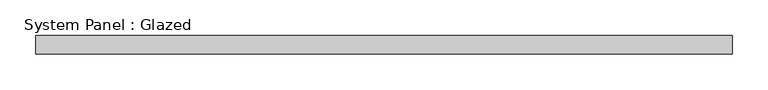
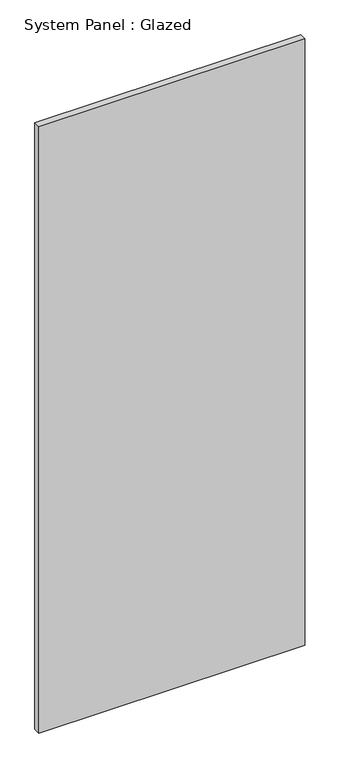
"""IFC4 building model written with IfcOpenShell, lengths in millimetres: plate geometry, System Panel : Glazed."""

from ifc_helpers import new_model, si_unit, origin, origin_with_axes, place, context, project, spatial, polyline, outline, extrude, source, transform, mapped, element, save


def system_panel_glazed_43d75c16(model_context):
    return source(origin(), model_context, "Body", "SweptSolid", [
        extrude(outline(polyline([(485.7750001, 19.05), (-485.7750001, 19.05), (-485.7750001, 44.45), (485.7750001, 44.45), (485.7750001, 19.05)])), origin_with_axes(), (0.0, 0.0, 1.0), 2343.15),
    ])


if __name__ == "__main__":
    model = new_model("IFC4")
    model_context = context("Model", 3, world=origin())
    ifc_project = project(units=[si_unit("LENGTHUNIT", "METRE", prefix="MILLI")], contexts=[model_context])
    site = spatial("IfcSite", under=ifc_project)
    building = spatial("IfcBuilding", under=site)
    placement = place(None, origin())
    system_panel_glazed_shape = system_panel_glazed_43d75c16(model_context)
    element("IfcPlate", 1, ObjectType="System Panel : Glazed", at=placement, inside=building, context=model_context, shape_type="MappedRepresentation", body=[
        mapped(system_panel_glazed_shape, transform((0.0, 0.0, 0.0), x_axis=(1.0, 0.0, 0.0), y_axis=(0.0, 1.0, 0.0), z_axis=(0.0, 0.0, 1.0))),
    ])
    save(model, "model.ifc")

# Revit data of these elements
# Type "System Panel : Glazed"
#   Construction Type Id = "GSP4R"
#   Analytic Construction = "1/8 in Pilkington single glazing"
#   Visual Light Transmittance = 0.9
#   Solar Heat Gain Coefficient = 0.86
#   Heat Transfer Coefficient (U) = 1.18115 BTU/(h·ft²·°F)
#   Define Thermal Properties by = 1
# Element 1 (IfcPlate, "System Panel : Glazed")
#   Materials on its faces: "Glass"
# Materials
#   "Glass": class "Glass", colour RGB 0 128 192, transparency 0.75, Description = "Soda Lime Glass", Cost = 0
